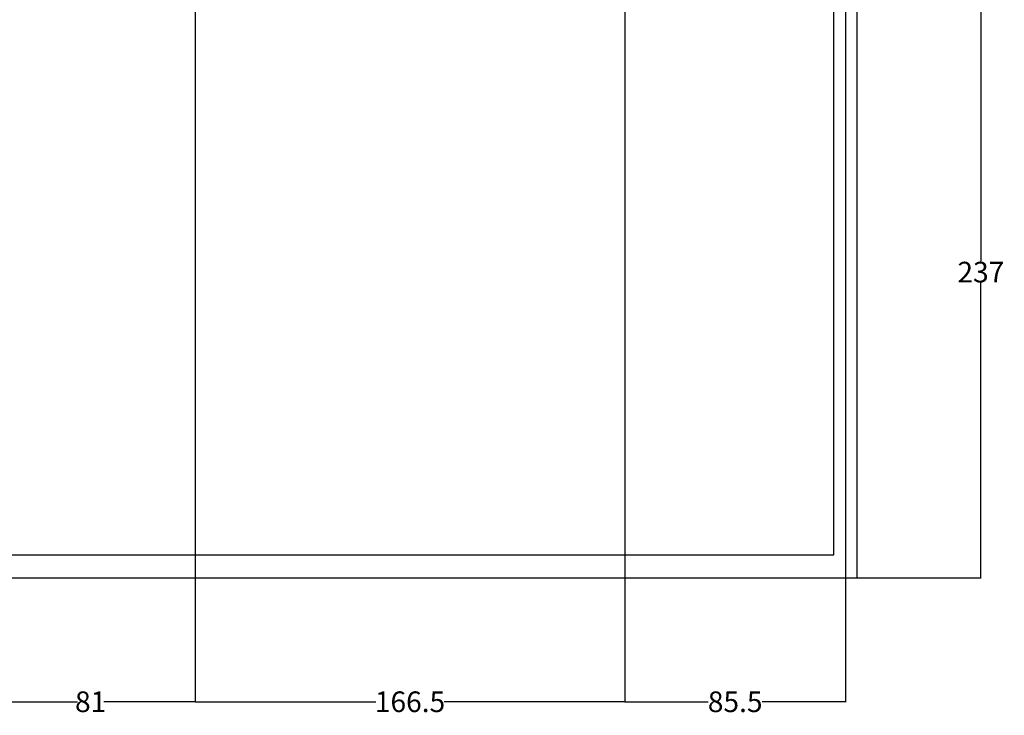
# Model space of a CAD drawing. Units: inches. Extents: x -48 to 50072, y 0 to 21068.
# Tile 62 of 75: x 974 to 1356, y 232 to 501. Entities that reach past the tile are written whole.
import ezdxf

# ---------------------------------------------------------------- set-up
doc = ezdxf.new("R2010")
doc.units = ezdxf.units.IN
doc.header["$MEASUREMENT"] = 0
doc.linetypes.add('ACAD_ISO02W100', pattern=[15, 12, -3])
for name, color, linetype, lineweight in [('A-ANNO-DIMS', 2, 'Continuous', 18), ('C-PROP', 7, 'Continuous', 25), ('C-PROP-REF', 32, 'ACAD_ISO02W100', 13)]:
    doc.layers.add(name, color=color, linetype=linetype, lineweight=lineweight)
doc.styles.get("Standard").update_dxf_attribs({"font": 'arial.ttf'})
doc.dimstyles.get("Standard").update_dxf_attribs({"dimtxt": 8, "dimasz": 0.18, "dimexe": 0.18, "dimexo": 0.0625, "dimgap": 0.09, "dimtad": 0, "dimtih": 1, "dimtoh": 1, "dimdec": 1, "dimzin": 0, "dimdsep": 46, "dimlunit": 4, "dimtxsty": 'Standard', "dimblk": 'ARCHTICK', "dimcen": 0.09, "dimadec": 0, "dimazin": 0, "dimtfac": 1, "dimtdec": 1, "dimtofl": 0, "dimtmove": 0, "dimatfit": 3, "dimldrblk": 'ARCHTICK', "dimfxl": 1, "dimtolj": 1, "dimtzin": 0, "dimarcsym": 0})

# ---------------------------------------------------------------- blocks, each defined once
blk = doc.blocks.new('_ArchTick')
at = {"color": 0, "linetype": 'ByBlock', "const_width": 0.15}
blk.add_lwpolyline([(-0.5, -0.5), (0.5, 0.5)], dxfattribs=at)
blk = doc.blocks.new('*D132')
at = {"layer": 'A-ANNO-DIMS', "color": 0, "lineweight": -2, "transparency": 16777216}
for p, q in [((1294.32, 521.76), (1346.89, 521.76)), ((1346.71, 521.76), (1346.71, 407.44)), ((1346.71, 284.76), (1346.71, 399.09)), ((1298.82, 284.76), (1346.89, 284.76))]:
    blk.add_line(p, q, dxfattribs=at)
at = {"layer": 'Defpoints', "color": 0, "transparency": 16777216}
for p in [(1294.26, 521.76), (1346.71, 521.76), (1298.76, 284.76)]:
    blk.add_point(p, dxfattribs=at)
at = {"layer": 'A-ANNO-DIMS', "color": 0, "lineweight": -2, "transparency": 16777216, "xscale": 0.18, "yscale": 0.18, "zscale": 0.18}
for p, rotation in [((1346.71, 521.76), 90), ((1346.71, 284.76), 270)]:
    blk.add_blockref('_ArchTick', p, dxfattribs=dict(at, rotation=rotation))
at = {"layer": 'A-ANNO-DIMS', "color": 0, "transparency": 16777216, "insert": (1346.71, 403.26), "char_height": 8, "attachment_point": 5}
blk.add_mtext('\\A1;237', dxfattribs=at)
blk = doc.blocks.new('*D137')
at = {"layer": 'A-ANNO-DIMS', "color": 0, "lineweight": -2, "transparency": 16777216}
for p, q in [((961.26, 559.4), (961.26, 236.63)), ((1042.26, 559.4), (1042.26, 236.63)), ((961.26, 236.81), (996.71, 236.81)), ((1042.26, 236.81), (1006.81, 236.81))]:
    blk.add_line(p, q, dxfattribs=at)
at = {"layer": 'Defpoints', "color": 0, "transparency": 16777216}
for p in [(961.26, 559.46), (1042.26, 559.46), (1042.26, 236.81)]:
    blk.add_point(p, dxfattribs=at)
at = {"layer": 'A-ANNO-DIMS', "color": 0, "lineweight": -2, "transparency": 16777216, "xscale": 0.18, "yscale": 0.18, "zscale": 0.18, "rotation": 180}
blk.add_blockref('_ArchTick', (961.26, 236.81), dxfattribs=at)
at = {"layer": 'A-ANNO-DIMS', "color": 0, "lineweight": -2, "transparency": 16777216, "xscale": 0.18, "yscale": 0.18, "zscale": 0.18}
blk.add_blockref('_ArchTick', (1042.26, 236.81), dxfattribs=at)
at = {"layer": 'A-ANNO-DIMS', "color": 0, "transparency": 16777216, "insert": (1001.76, 236.81), "char_height": 8, "attachment_point": 5}
blk.add_mtext('\\A1;81', dxfattribs=at)
blk = doc.blocks.new('*D138')
at = {"layer": 'A-ANNO-DIMS', "color": 0, "lineweight": -2, "transparency": 16777216}
for p, q in [((1042.26, 559.4), (1042.26, 236.63)), ((1208.76, 559.4), (1208.76, 236.63)), ((1042.26, 236.81), (1112.27, 236.81)), ((1208.76, 236.81), (1138.75, 236.81))]:
    blk.add_line(p, q, dxfattribs=at)
at = {"layer": 'Defpoints', "color": 0, "transparency": 16777216}
for p in [(1042.26, 559.46), (1208.76, 559.46), (1208.76, 236.81)]:
    blk.add_point(p, dxfattribs=at)
at = {"layer": 'A-ANNO-DIMS', "color": 0, "lineweight": -2, "transparency": 16777216, "xscale": 0.18, "yscale": 0.18, "zscale": 0.18, "rotation": 180}
blk.add_blockref('_ArchTick', (1042.26, 236.81), dxfattribs=at)
at = {"layer": 'A-ANNO-DIMS', "color": 0, "lineweight": -2, "transparency": 16777216, "xscale": 0.18, "yscale": 0.18, "zscale": 0.18}
blk.add_blockref('_ArchTick', (1208.76, 236.81), dxfattribs=at)
at = {"layer": 'A-ANNO-DIMS', "color": 0, "transparency": 16777216, "insert": (1125.51, 236.81), "char_height": 8, "attachment_point": 5}
blk.add_mtext('\\A1;166.5', dxfattribs=at)
blk = doc.blocks.new('*D139')
at = {"layer": 'A-ANNO-DIMS', "color": 0, "lineweight": -2, "transparency": 16777216}
for p, q in [((1208.76, 530.7), (1208.76, 236.63)), ((1294.26, 521.7), (1294.26, 236.63)), ((1208.76, 236.81), (1241, 236.81)), ((1294.26, 236.81), (1262.03, 236.81))]:
    blk.add_line(p, q, dxfattribs=at)
at = {"layer": 'Defpoints', "color": 0, "transparency": 16777216}
for p in [(1208.76, 530.76), (1294.26, 521.76), (1294.26, 236.81)]:
    blk.add_point(p, dxfattribs=at)
at = {"layer": 'A-ANNO-DIMS', "color": 0, "lineweight": -2, "transparency": 16777216, "xscale": 0.18, "yscale": 0.18, "zscale": 0.18, "rotation": 180}
blk.add_blockref('_ArchTick', (1208.76, 236.81), dxfattribs=at)
at = {"layer": 'A-ANNO-DIMS', "color": 0, "lineweight": -2, "transparency": 16777216, "xscale": 0.18, "yscale": 0.18, "zscale": 0.18}
blk.add_blockref('_ArchTick', (1294.26, 236.81), dxfattribs=at)
at = {"layer": 'A-ANNO-DIMS', "color": 0, "transparency": 16777216, "insert": (1251.51, 236.81), "char_height": 8, "attachment_point": 5}
blk.add_mtext('\\A1;85.5', dxfattribs=at)

msp = doc.modelspace()

# ---------------------------------------------------------------- linework, layer by layer
at = {"layer": 'C-PROP'}
for p, q in [((1298.761, 284.764), (1298.761, 1241.464)), ((1289.761, 293.764), (1289.761, 559.464)), ((767.761, 293.764), (1289.761, 293.764)), ((758.761, 284.764), (1298.761, 284.764))]:
    msp.add_line(p, q, dxfattribs=at)
at = {"layer": 'C-PROP-REF'}
msp.add_line((1294.261, 284.764), (1294.261, 1236.964), dxfattribs=at)

# ---------------------------------------------------------------- dimensions: what is measured, and where the dimension line sits
at = {"layer": 'A-ANNO-DIMS'}
for base, p1, p2, override, picture, middle in [((1042.261, 236.814), (961.261, 559.464), (1042.261, 559.464), {"dimdec": 0, "dimlfac": 1, "dimrnd": 0, "dimzin": 0, "dimdsep": 46, "dimlunit": 2}, '*D137', (1001.761, 236.814)), ((1208.761, 236.814), (1042.261, 559.464), (1208.761, 559.464), {"dimdec": 1, "dimlfac": 1, "dimrnd": 0, "dimzin": 0, "dimdsep": 46, "dimlunit": 2}, '*D138', (1125.511, 236.814)), ((1294.261, 236.814), (1208.761, 530.764), (1294.261, 521.764), {"dimdec": 1, "dimlfac": 1, "dimrnd": 0, "dimzin": 0, "dimdsep": 46, "dimlunit": 2}, '*D139', (1251.511, 236.814))]:
    dim = msp.add_linear_dim(base=base, p1=p1, p2=p2, dimstyle='Standard', override=override, dxfattribs=at)
    dim.commit()
    dim.dimension.update_dxf_attribs({"geometry": picture, "text_midpoint": middle})
dim = msp.add_linear_dim(base=(1346.711, 521.764), p1=(1298.761, 284.764), p2=(1294.261, 521.764), angle=90, dimstyle='Standard', override={"dimdec": 0, "dimlfac": 1, "dimrnd": 0, "dimzin": 0, "dimdsep": 46, "dimlunit": 2}, dxfattribs=at)
dim.commit()
dim.dimension.update_dxf_attribs({"geometry": '*D132', "text_midpoint": (1346.711, 403.264)})

doc.saveas('drawing.dxf')
